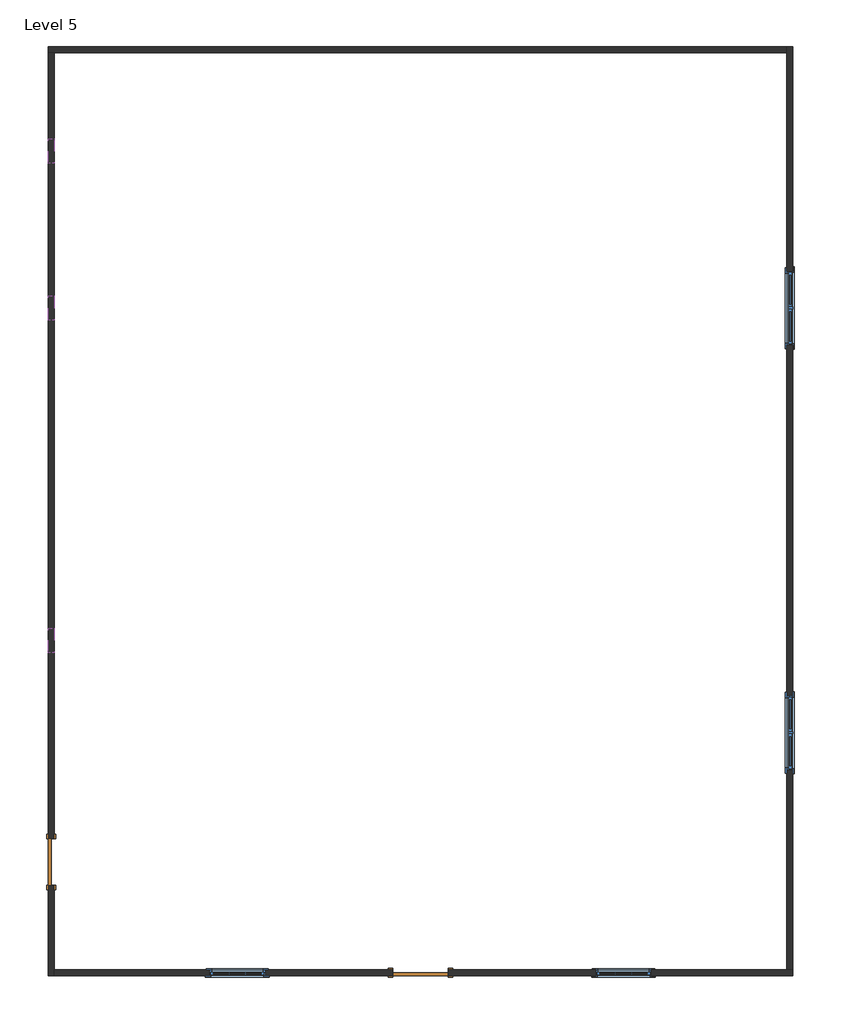
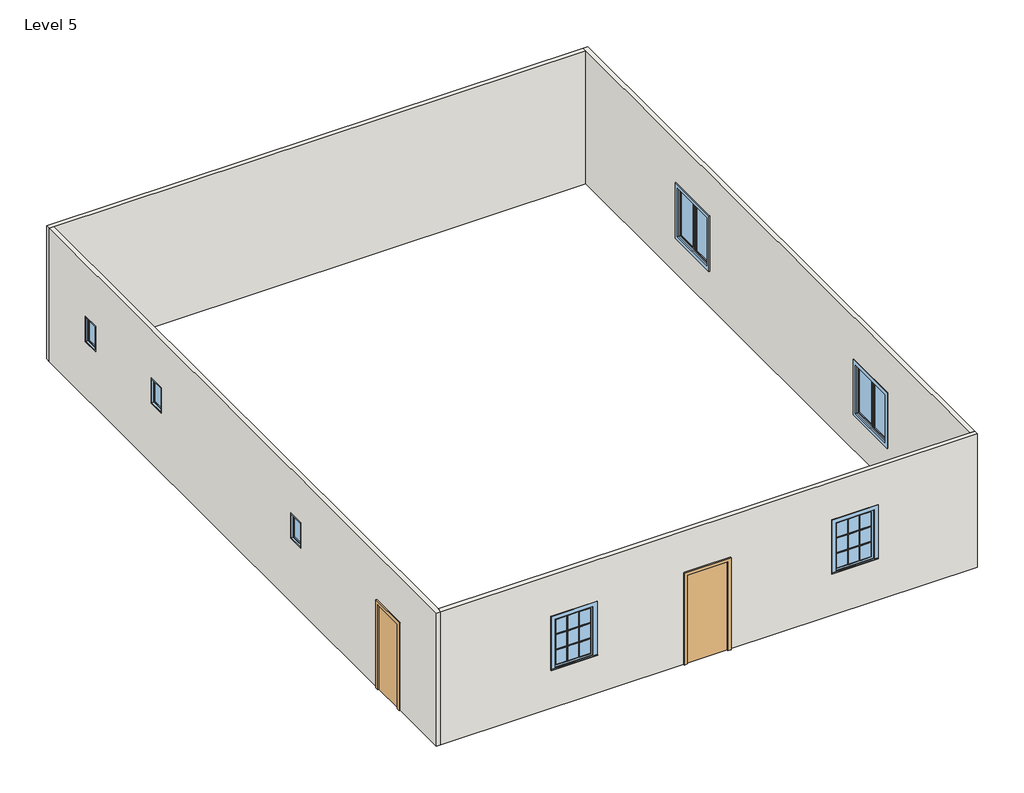
# One storey, incomplete: 7 windows, 4 walls, 2 doors.
"""IFC4 building model written with IfcOpenShell, lengths in millimetres."""

from ifc_helpers import new_model, si_unit, origin, place, context, project, spatial, faceted_brep, transform, mapped, element, save
from components import door_29583826, door_048588e9, window_ad8769eb, window_90ef9153, window_a112695e

model = new_model("IFC4")

# Units and contexts
model_context = context("Model", 3, world=origin())
ifc_project = project(units=[si_unit("LENGTHUNIT", "METRE", prefix="MILLI")], contexts=[model_context])

# Site, building, storey
site = spatial("IfcSite", under=ifc_project)
building = spatial("IfcBuilding", under=site)
storey = spatial("IfcBuildingStorey", under=building, Name="Level 5", Elevation=6400.8)

# Doors
placement = place(None, origin())
door_shape = door_29583826(model_context)
element("IfcDoor", 1, ObjectType="Single-Flush : 30\" x 80\"", at=placement, inside=storey, context=model_context, shape_type="MappedRepresentation", body=[
    mapped(door_shape, transform((1744.5168112, -162.0718204, 6400.8), x_axis=(0.0, 1.0, 0.0), y_axis=(-1.0, 0.0, 0.0), z_axis=(0.0, 0.0, 1.0))),
])
door_2_shape = door_048588e9(model_context)
element("IfcDoor", 2, ObjectType="Single-Flush : 36\" x 84\"", at=placement, inside=storey, context=model_context, shape_type="MappedRepresentation", body=[
    mapped(door_2_shape, transform((7840.5168112, -1990.8718204, 6400.8), x_axis=(-1.0, 0.0, 0.0), y_axis=(0.0, -1.0, 0.0), z_axis=(0.0, 0.0, 1.0))),
])

# Walls
element("IfcWall", 3, ObjectType="Generic - 4\" Brick", at=placement, inside=storey, context=model_context, shape_type="Brep", body=[
    faceted_brep([(1693.7168112, 13198.3281796, 6400.8), (1795.3168112, 13198.3281796, 6400.8), (13885.7168112, 13198.3281796, 6400.8), (13885.7168112, 13198.3281796, 9601.2), (1795.3168112, 13198.3281796, 9601.2), (1693.7168112, 13198.3281796, 9601.2), (1693.7168112, 13299.9281796, 6400.8), (1693.7168112, 13299.9281796, 9601.2), (13885.7168112, 13299.9281796, 9601.2), (13885.7168112, 13299.9281796, 6400.8)], [[[0, 1, 2, 3, 4, 5]], [[6, 7, 8, 9]], [[2, 1, 0, 6, 9]], [[0, 5, 7, 6]], [[3, 2, 9, 8]], [[5, 4, 3, 8, 7]]]),
])
element("IfcWall", 4, ObjectType="Generic - 4\" Brick", at=placement, inside=storey, context=model_context, shape_type="Brep", body=[
    faceted_brep([(1795.3168112, 218.9281796, 8432.8), (1795.3168112, 218.9281796, 6400.8), (1795.3168112, 13198.3281796, 6400.8), (1795.3168112, 13198.3281796, 9601.2), (1795.3168112, -1940.0718204, 9601.2), (1795.3168112, -2041.6718204, 9601.2), (1795.3168112, -2041.6718204, 6400.8), (1795.3168112, -1940.0718204, 6400.8), (1795.3168112, -543.0718204, 6400.8), (1795.3168112, -543.0718204, 8432.8), (1795.3168112, 8778.7281796, 8445.3590075), (1795.3168112, 9185.1281796, 8445.3590075), (1795.3168112, 9185.1281796, 7835.7590075), (1795.3168112, 8778.7281796, 7835.7590075), (1795.3168112, 11369.5281796, 8351.5224411), (1795.3168112, 11775.9281796, 8351.5224411), (1795.3168112, 11775.9281796, 7741.9224411), (1795.3168112, 11369.5281796, 7741.9224411), (1795.3168112, 3292.3281796, 8529.2575158), (1795.3168112, 3698.7281796, 8529.2575158), (1795.3168112, 3698.7281796, 7919.6575158), (1795.3168112, 3292.3281796, 7919.6575158), (1693.7168112, 13198.3281796, 6400.8), (1693.7168112, 218.9281796, 6400.8), (1693.7168112, 218.9281796, 8432.8), (1693.7168112, -543.0718204, 8432.8), (1693.7168112, -543.0718204, 6400.8), (1693.7168112, -2041.6718204, 6400.8), (1693.7168112, -2041.6718204, 9601.2), (1693.7168112, 13198.3281796, 9601.2), (1693.7168112, 8778.7281796, 8445.3590075), (1693.7168112, 8778.7281796, 7835.7590075), (1693.7168112, 9185.1281796, 7835.7590075), (1693.7168112, 9185.1281796, 8445.3590075), (1693.7168112, 11369.5281796, 8351.5224411), (1693.7168112, 11369.5281796, 7741.9224411), (1693.7168112, 11775.9281796, 7741.9224411), (1693.7168112, 11775.9281796, 8351.5224411), (1693.7168112, 3292.3281796, 8529.2575158), (1693.7168112, 3292.3281796, 7919.6575158), (1693.7168112, 3698.7281796, 7919.6575158), (1693.7168112, 3698.7281796, 8529.2575158)], [[[0, 1, 2, 3, 4, 5, 6, 7, 8, 9], [10, 11, 12, 13], [14, 15, 16, 17], [18, 19, 20, 21]], [[22, 23, 24, 25, 26, 27, 28, 29], [30, 31, 32, 33], [34, 35, 36, 37], [38, 39, 40, 41]], [[2, 1, 23, 22]], [[8, 7, 6, 27, 26]], [[6, 5, 28, 27]], [[3, 2, 22, 29]], [[5, 4, 3, 29, 28]], [[24, 23, 1, 0]], [[25, 24, 0, 9]], [[26, 25, 9, 8]], [[31, 30, 10, 13]], [[32, 31, 13, 12]], [[33, 32, 12, 11]], [[30, 33, 11, 10]], [[35, 34, 14, 17]], [[36, 35, 17, 16]], [[37, 36, 16, 15]], [[34, 37, 15, 14]], [[39, 38, 18, 21]], [[40, 39, 21, 20]], [[41, 40, 20, 19]], [[38, 41, 19, 18]]]),
])
element("IfcWall", 5, ObjectType="Generic - 4\" Brick", at=placement, inside=storey, context=model_context, shape_type="Brep", body=[
    faceted_brep([(7383.3168112, -1940.0718204, 8534.4), (7383.3168112, -1940.0718204, 6400.8), (1795.3168112, -1940.0718204, 6400.8), (1795.3168112, -1940.0718204, 9601.2), (13885.7168112, -1940.0718204, 9601.2), (13987.3168112, -1940.0718204, 9601.2), (13987.3168112, -1940.0718204, 6400.8), (13885.7168112, -1940.0718204, 6400.8), (8297.7168112, -1940.0718204, 6400.8), (8297.7168112, -1940.0718204, 8534.4), (4360.7168112, -1940.0718204, 8540.8896063), (4360.7168112, -1940.0718204, 7321.6896063), (5275.1168112, -1940.0718204, 7321.6896063), (5275.1168112, -1940.0718204, 8540.8896063), (10736.1168112, -1940.0718204, 8627.178551), (10736.1168112, -1940.0718204, 7407.978551), (11650.5168112, -1940.0718204, 7407.978551), (11650.5168112, -1940.0718204, 8627.178551), (1795.3168112, -2041.6718204, 6400.8), (7383.3168112, -2041.6718204, 6400.8), (7383.3168112, -2041.6718204, 8534.4), (8297.7168112, -2041.6718204, 8534.4), (8297.7168112, -2041.6718204, 6400.8), (13987.3168112, -2041.6718204, 6400.8), (13987.3168112, -2041.6718204, 9601.2), (1795.3168112, -2041.6718204, 9601.2), (4360.7168112, -2041.6718204, 8540.8896063), (5275.1168112, -2041.6718204, 8540.8896063), (5275.1168112, -2041.6718204, 7321.6896063), (4360.7168112, -2041.6718204, 7321.6896063), (10736.1168112, -2041.6718204, 8627.178551), (11650.5168112, -2041.6718204, 8627.178551), (11650.5168112, -2041.6718204, 7407.978551), (10736.1168112, -2041.6718204, 7407.978551)], [[[0, 1, 2, 3, 4, 5, 6, 7, 8, 9], [10, 11, 12, 13], [14, 15, 16, 17]], [[18, 19, 20, 21, 22, 23, 24, 25], [26, 27, 28, 29], [30, 31, 32, 33]], [[2, 1, 19, 18]], [[8, 7, 6, 23, 22]], [[6, 5, 24, 23]], [[3, 2, 18, 25]], [[5, 4, 3, 25, 24]], [[20, 19, 1, 0]], [[21, 20, 0, 9]], [[22, 21, 9, 8]], [[11, 10, 26, 29]], [[12, 11, 29, 28]], [[13, 12, 28, 27]], [[10, 13, 27, 26]], [[15, 14, 30, 33]], [[16, 15, 33, 32]], [[17, 16, 32, 31]], [[14, 17, 31, 30]]]),
])
element("IfcWall", 6, ObjectType="Generic - 4\" Brick", at=placement, inside=storey, context=model_context, shape_type="Brep", body=[
    faceted_brep([(13885.7168112, 13299.9281796, 6400.8), (13885.7168112, 13198.3281796, 6400.8), (13885.7168112, -1940.0718204, 6400.8), (13885.7168112, -1940.0718204, 9601.2), (13885.7168112, 13198.3281796, 9601.2), (13885.7168112, 13299.9281796, 9601.2), (13885.7168112, 8372.3281796, 8534.4), (13885.7168112, 8372.3281796, 7315.2), (13885.7168112, 9591.5281796, 7315.2), (13885.7168112, 9591.5281796, 8534.4), (13885.7168112, 1361.9281796, 8534.4), (13885.7168112, 1361.9281796, 7315.2), (13885.7168112, 2581.1281796, 7315.2), (13885.7168112, 2581.1281796, 8534.4), (13987.3168112, 13299.9281796, 6400.8), (13987.3168112, 13299.9281796, 9601.2), (13987.3168112, -1940.0718204, 9601.2), (13987.3168112, -1940.0718204, 6400.8), (13987.3168112, 8372.3281796, 8534.4), (13987.3168112, 9591.5281796, 8534.4), (13987.3168112, 9591.5281796, 7315.2), (13987.3168112, 8372.3281796, 7315.2), (13987.3168112, 1361.9281796, 8534.4), (13987.3168112, 2581.1281796, 8534.4), (13987.3168112, 2581.1281796, 7315.2), (13987.3168112, 1361.9281796, 7315.2)], [[[0, 1, 2, 3, 4, 5], [6, 7, 8, 9], [10, 11, 12, 13]], [[14, 15, 16, 17], [18, 19, 20, 21], [22, 23, 24, 25]], [[2, 1, 0, 14, 17]], [[0, 5, 15, 14]], [[3, 2, 17, 16]], [[5, 4, 3, 16, 15]], [[7, 6, 18, 21]], [[8, 7, 21, 20]], [[9, 8, 20, 19]], [[6, 9, 19, 18]], [[11, 10, 22, 25]], [[12, 11, 25, 24]], [[13, 12, 24, 23]], [[10, 13, 23, 22]]]),
])

# Windows
window_shape = window_ad8769eb(model_context)
element("IfcWindow", 7, ObjectType="Casement 3x3 with Trim : 36\" x 48\"", at=placement, inside=storey, context=model_context, shape_type="MappedRepresentation", body=[
    mapped(window_shape, transform((4817.9168112, -1990.8718204, 6407.2896063), x_axis=(-1.0, 0.0, 0.0), y_axis=(0.0, -1.0, 0.0), z_axis=(0.0, 0.0, 1.0))),
])
element("IfcWindow", 8, ObjectType="Casement 3x3 with Trim : 36\" x 48\"", at=placement, inside=storey, context=model_context, shape_type="MappedRepresentation", body=[
    mapped(window_shape, transform((11193.3168112, -1990.8718204, 6493.578551), x_axis=(-1.0, 0.0, 0.0), y_axis=(0.0, -1.0, 0.0), z_axis=(0.0, 0.0, 1.0))),
])
window_2_shape = window_90ef9153(model_context)
element("IfcWindow", 9, ObjectType="Casement Dbl with Trim : 48\" x 48\"", at=placement, inside=storey, context=model_context, shape_type="MappedRepresentation", body=[
    mapped(window_2_shape, transform((13917.4668112, 8981.9281796, 6400.8), x_axis=(0.0, -1.0, 0.0), y_axis=(1.0, 0.0, 0.0), z_axis=(0.0, 0.0, 1.0))),
])
element("IfcWindow", 10, ObjectType="Casement Dbl with Trim : 48\" x 48\"", at=placement, inside=storey, context=model_context, shape_type="MappedRepresentation", body=[
    mapped(window_2_shape, transform((13917.4668112, 1971.5281796, 6400.8), x_axis=(0.0, -1.0, 0.0), y_axis=(1.0, 0.0, 0.0), z_axis=(0.0, 0.0, 1.0))),
])
window_3_shape = window_a112695e(model_context)
element("IfcWindow", 11, ObjectType="Fixed : 16\" x 24\"", at=placement, inside=storey, context=model_context, shape_type="MappedRepresentation", body=[
    mapped(window_3_shape, transform((1744.5168112, 8943.8281796, 6921.3590075), x_axis=(0.0, -1.0, 0.0), y_axis=(1.0, 0.0, 0.0), z_axis=(0.0, 0.0, 1.0))),
])
element("IfcWindow", 12, ObjectType="Fixed : 16\" x 24\"", at=placement, inside=storey, context=model_context, shape_type="MappedRepresentation", body=[
    mapped(window_3_shape, transform((1744.5168112, 11534.6281796, 6827.5224411), x_axis=(0.0, -1.0, 0.0), y_axis=(1.0, 0.0, 0.0), z_axis=(0.0, 0.0, 1.0))),
])
element("IfcWindow", 13, ObjectType="Fixed : 16\" x 24\"", at=placement, inside=storey, context=model_context, shape_type="MappedRepresentation", body=[
    mapped(window_3_shape, transform((1744.5168112, 3457.4281796, 7005.2575158), x_axis=(0.0, -1.0, 0.0), y_axis=(1.0, 0.0, 0.0), z_axis=(0.0, 0.0, 1.0))),
])

save(model, "model.ifc")

# Revit data of these elements
# Type "Single-Flush : 30\" x 80\""
#   Type Mark = "5"
#   Construction Type Id = "MDOOR"
#   Assembly Code = "C1020"
#   Analytic Construction = "Metal"
#   Thickness = 0' - 2"
#   Heat Transfer Coefficient (U) = 0.651978 BTU/(h·ft²·°F)
#   Height = 6' - 8"
#   Trim Projection Ext = 0' - 1"
#   Trim Projection Int = 0' - 1"
#   Trim Width = 0' - 3"
#   Width = 2' - 6"
#   Define Thermal Properties by = 1
#   Door Material = Door - Panel
#   Frame Material = Door - Frame
#   Visual Light Transmittance = 0
#   Solar Heat Gain Coefficient = 0
#   Function = (empty or 0)
#   Wall Closure = (empty or 0)
# Type "Single-Flush : 36\" x 84\""
#   Type Mark = "1"
#   Construction Type Id = "MDOOR"
#   Assembly Code = "C1020"
#   Analytic Construction = "Metal"
#   Thickness = 0' - 2"
#   Heat Transfer Coefficient (U) = 0.651978 BTU/(h·ft²·°F)
#   Height = 7' - 0"
#   Trim Projection Ext = 0' - 1"
#   Trim Projection Int = 0' - 1"
#   Trim Width = 0' - 3"
#   Width = 3' - 0"
#   Define Thermal Properties by = 1
#   Door Material = Door - Panel
#   Frame Material = Door - Frame
#   Visual Light Transmittance = 0
#   Solar Heat Gain Coefficient = 0
#   Function = (empty or 0)
#   Wall Closure = (empty or 0)
# Type "Generic - 4\" Brick"
#   Assembly Code = "B2010"
#   Layers, outside or top first: 0' - 4" "Brick, Common" (function 1)
# Type "Casement 3x3 with Trim : 36\" x 48\""
#   Type Mark = "10"
#   Construction Type Id = "GSP4R"
#   Assembly Code = "B2020100"
#   Analytic Construction = "1/8 in Pilkington single glazing"
#   Visual Light Transmittance = 0.9
#   Solar Heat Gain Coefficient = 0.78
#   Heat Transfer Coefficient (U) = 0.6496 BTU/(h·ft²·°F)
#   Height = 4' - 0"
#   Default Sill Height = 3' - 0"
#   Trim Projection - Ext. = 0' - 0 1/2"
#   Trim Projection - Int. = 0' - 0 3/4"
#   Trim Width - Exterior = 0' - 3 1/2"
#   Trim Width - Interior = 0' - 3 1/2"
#   Width = 3' - 0"
#   Window Inset = 0' - 0 3/4"
#   Define Thermal Properties by = 1
#   Glass Pane Material = Glass
#   Sash Material = Sash
#   Trim Exterior Material = Trim
#   Trim Interior Material = Trim
#   Wall Closure = (empty or 0)
# Type "Casement Dbl with Trim : 48\" x 48\""
#   Type Mark = "13"
#   Construction Type Id = "GSP4R"
#   Assembly Code = "B2020100"
#   Analytic Construction = "1/8 in Pilkington single glazing"
#   Visual Light Transmittance = 0.9
#   Solar Heat Gain Coefficient = 0.78
#   Heat Transfer Coefficient (U) = 0.6496 BTU/(h·ft²·°F)
#   Height = 4' - 0"
#   Default Sill Height = 3' - 0"
#   Trim Projection - Ext. = 0' - 0 1/2"
#   Trim Projection - Int. = 0' - 0 3/4"
#   Trim Width - Exterior = 0' - 3 1/2"
#   Trim Width - Interior = 0' - 3 1/2"
#   Width = 4' - 0"
#   Window Inset = 0' - 0 3/4"
#   Define Thermal Properties by = 1
#   Glass Pane Material = Glass
#   Sash Material = Sash
#   Trim Exterior Material = Trim
#   Trim Interior Material = Trim
#   Wall Closure = (empty or 0)
# Type "Fixed : 16\" x 24\""
#   Type Mark = "4"
#   Construction Type Id = "GSP4R"
#   Assembly Code = "B2020100"
#   Analytic Construction = "1/8 in Pilkington single glazing"
#   Visual Light Transmittance = 0.9
#   Solar Heat Gain Coefficient = 0.78
#   Heat Transfer Coefficient (U) = 0.6496 BTU/(h·ft²·°F)
#   Height = 2' - 0"
#   Default Sill Height = 3' - 0"
#   Width = 1' - 4"
#   Window Inset = 0' - 0 3/4"
#   Define Thermal Properties by = 1
#   Glass Pane Material = Glass
#   Sash Material = Sash
#   Wall Closure = (empty or 0)
# Element 1 (IfcDoor, "Single-Flush : 30\" x 80\"")
#   Phase Created = New Construction
#   Materials on its faces: "Door - Frame", "Door - Panel"
# Element 2 (IfcDoor, "Single-Flush : 36\" x 84\"")
#   Phase Created = New Construction
#   Materials on its faces: "Door - Frame", "Door - Panel"
# Elements 3, 4, 5, 6 (IfcWall, "Generic - 4\" Brick")
#   Top Offset = 0' - 0"
#   Base Offset = 0' - 0"
#   Unconnected Height = 10' - 0"
#   wall height = 10' - 0"
#   Phase Created = New Construction
#   Base Constraint = Level 5
#   Materials on its faces: "Brick, Common"
# Element 7 (IfcWindow, "Casement 3x3 with Trim : 36\" x 48\"")
#   Mark = "17"
#   Phase Created = New Construction
#   Materials on its faces: "Sash", "Glass", "Trim"
# Element 8 (IfcWindow, "Casement 3x3 with Trim : 36\" x 48\"")
#   Mark = "18"
#   Phase Created = New Construction
#   Materials on its faces: "Sash", "Glass", "Trim"
# Element 9 (IfcWindow, "Casement Dbl with Trim : 48\" x 48\"")
#   Mark = "25"
#   Phase Created = New Construction
#   Materials on its faces: "Sash", "Trim", "Glass"
# Element 10 (IfcWindow, "Casement Dbl with Trim : 48\" x 48\"")
#   Mark = "26"
#   Phase Created = New Construction
#   Materials on its faces: "Sash", "Trim", "Glass"
# Element 11 (IfcWindow, "Fixed : 16\" x 24\"")
#   Mark = "5"
#   Phase Created = New Construction
#   Materials on its faces: "Sash", "Glass"
# Element 12 (IfcWindow, "Fixed : 16\" x 24\"")
#   Mark = "6"
#   Phase Created = New Construction
#   Materials on its faces: "Sash", "Glass"
# Element 13 (IfcWindow, "Fixed : 16\" x 24\"")
#   Mark = "11"
#   Phase Created = New Construction
#   Materials on its faces: "Sash", "Glass"
# Materials
#   "Door - Panel": class "Wood", colour RGB 210 159 95, transparency 0
#   "Door - Frame": colour RGB 118 70 51, transparency 0
#   "Brick, Common": class "Masonry", colour RGB 170 98 104, transparency 0, Description = "Common brick", Cost = 0
#   "Glass": class "Glass", colour RGB 0 128 192, transparency 0.75, Description = "Soda Lime Glass", Cost = 0
#   "Sash": class "Wood", colour RGB 224 178 126, transparency 0
#   "Trim": class "Wood", colour RGB 224 178 126, transparency 0
